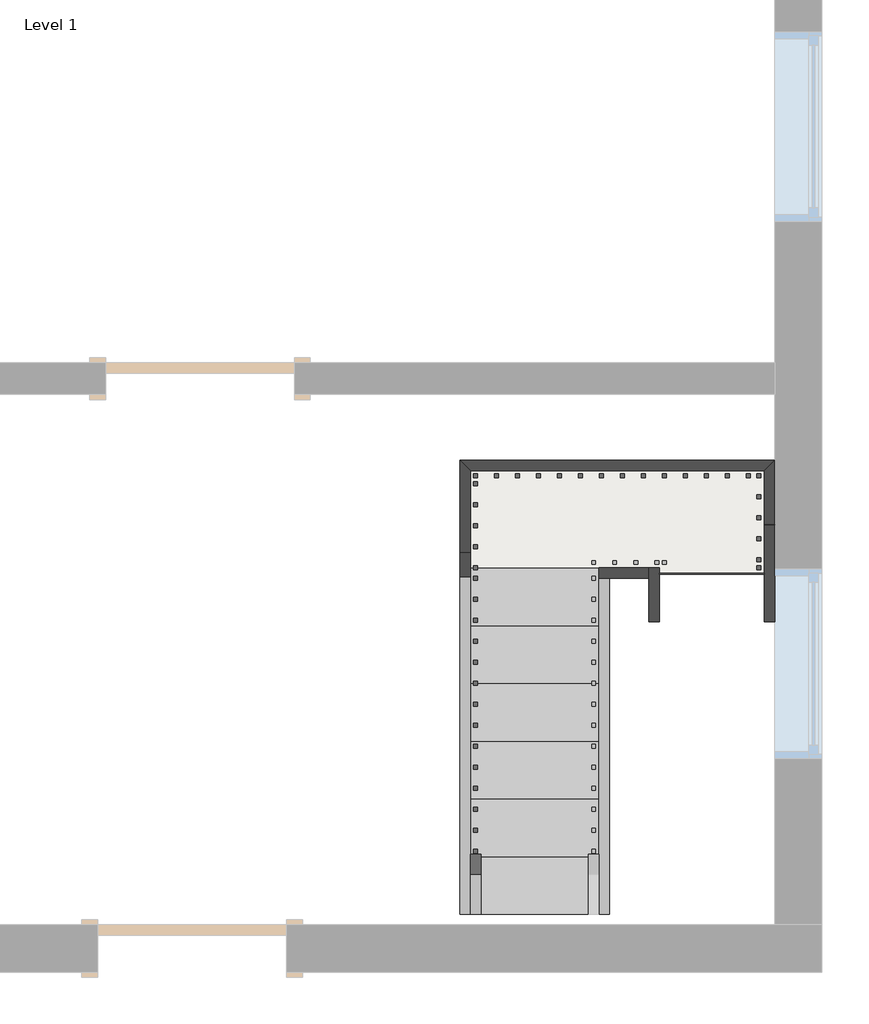
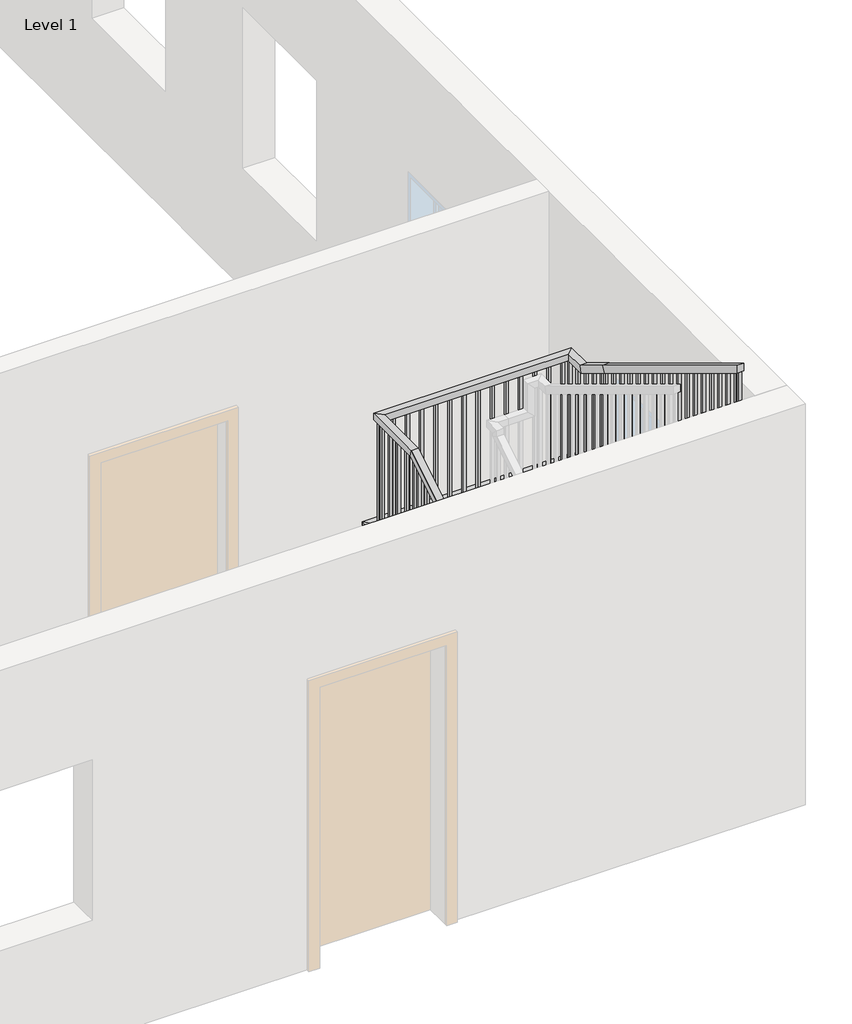
# One storey, part 2 of 2: 8 members, 2 stair flights, 1 railing, 1 slab.
"""IFC4 building model written with IfcOpenShell, lengths in millimetres."""

from ifc_helpers import new_model, si_unit, frame, origin, place, context, project, spatial, polyline, outline, extrude, faceted_brep, transform, mapped, element, save
from components import non_monolithic_landing_1ef36e8a, stair_flight_33de849b, stair_flight_7fe2dcbd

model = new_model("IFC4")

# Units and contexts
model_context = context("Model", 3, world=origin())
ifc_project = project(units=[si_unit("LENGTHUNIT", "METRE", prefix="MILLI")], contexts=[model_context])

# Site, building, storey
site = spatial("IfcSite", under=ifc_project)
building = spatial("IfcBuilding", under=site)
storey = spatial("IfcBuildingStorey", under=building, Name="Level 1", Elevation=0.0)

# Members
placement = place(None, origin())
element("IfcMember", 1, ObjectType="Stringer - 2\" Width", at=placement, inside=storey, context=model_context, shape_type="SweptSolid", body=[
    extrude(outline(polyline([(-4479.3424149, 0.0), (-4479.3424149, 212.114512), (-2747.8013597, 1261.5333333), (-2662.6469032, 956.7333333), (-4241.2569032, 0.0), (-4479.3424149, 0.0)])), frame((-1585.4629117, 0.0, 0.0), z_axis=(1.0, 0.0, 0.0), x_axis=(0.0, 1.0, 0.0)), (0.0, 0.0, 1.0), 50.8),
])
element("IfcMember", 2, ObjectType="Stringer - 2\" Width", at=placement, inside=storey, context=model_context, shape_type="SweptSolid", body=[
    extrude(outline(polyline([(-4479.3424149, 0.0), (-4479.3424149, 212.114512), (-2853.7424149, 1197.3266332), (-2853.7424149, 840.9178717), (-4241.2569032, 0.0), (-4479.3424149, 0.0)])), frame((-912.3629117, 0.0, 0.0), z_axis=(1.0, 0.0, 0.0), x_axis=(0.0, 1.0, 0.0)), (0.0, 0.0, 1.0), 50.8),
])
element("IfcMember", 3, ObjectType="Stringer - 2\" Width", at=placement, inside=storey, context=model_context, shape_type="SweptSolid", body=[
    extrude(outline(polyline([(-2578.6834702, 1261.5333333), (-2663.8379267, 956.7333333), (-4479.3424149, 2057.0390838), (-4479.3424149, 2413.4478453), (-2578.6834702, 1261.5333333)])), frame((-112.2629117, 0.0, 0.0), z_axis=(1.0, 0.0, 0.0), x_axis=(0.0, 1.0, 0.0)), (0.0, 0.0, 1.0), 50.8),
])
element("IfcMember", 4, ObjectType="Stringer - 2\" Width", at=placement, inside=storey, context=model_context, shape_type="SweptSolid", body=[
    extrude(outline(polyline([(-2802.9424149, 1397.4478453), (-2802.9424149, 1041.0390838), (-4479.3424149, 2057.0390838), (-4479.3424149, 2413.4478453), (-2802.9424149, 1397.4478453)])), frame((-671.0629117, 0.0, 0.0), z_axis=(1.0, 0.0, 0.0), x_axis=(0.0, 1.0, 0.0)), (0.0, 0.0, 1.0), 50.8),
])
element("IfcMember", 5, ObjectType="Stringer - 2\" Width", at=placement, inside=storey, context=model_context, shape_type="Brep", body=[
    faceted_brep([(-112.2629117, -2578.6834702, 1261.5333333), (-61.4629117, -2578.6834702, 1261.5333333), (-61.4629117, -2282.2424149, 1261.5333333), (-112.2629117, -2333.0424149, 1261.5333333), (-112.2629117, -2663.8379267, 956.7333333), (-112.2629117, -2333.0424149, 956.7333333), (-61.4629117, -2663.8379267, 956.7333333), (-61.4629117, -2282.2424149, 956.7333333)], [[[0, 1, 2, 3]], [[4, 0, 3, 5]], [[6, 4, 5, 7]], [[1, 6, 7, 2]], [[1, 0, 4, 6]], [[2, 7, 5, 3]]]),
])
element("IfcMember", 6, ObjectType="Stringer - 2\" Width", at=placement, inside=storey, context=model_context, shape_type="SweptSolid", body=[
    extrude(outline(polyline([(-61.4629117, -2282.2424149), (-112.2629117, -2333.0424149), (-1534.6629117, -2333.0424149), (-1585.4629117, -2282.2424149), (-61.4629117, -2282.2424149)])), frame((0.0, 0.0, 956.7333333), z_axis=(0.0, 0.0, 1.0), x_axis=(1.0, 0.0, 0.0)), (0.0, 0.0, 1.0), 304.8),
])
element("IfcMember", 7, ObjectType="Stringer - 2\" Width", at=placement, inside=storey, context=model_context, shape_type="Brep", body=[
    faceted_brep([(-1534.6629117, -2333.0424149, 1261.5333333), (-1585.4629117, -2282.2424149, 1261.5333333), (-1585.4629117, -2747.8013597, 1261.5333333), (-1534.6629117, -2747.8013597, 1261.5333333), (-1534.6629117, -2333.0424149, 956.7333333), (-1534.6629117, -2662.6469032, 956.7333333), (-1585.4629117, -2282.2424149, 956.7333333), (-1585.4629117, -2662.6469032, 956.7333333)], [[[0, 1, 2, 3]], [[4, 0, 3, 5]], [[6, 4, 5, 7]], [[1, 6, 7, 2]], [[1, 0, 4, 6]], [[2, 7, 5, 3]]]),
])
element("IfcMember", 8, ObjectType="Stringer - 2\" Width", at=placement, inside=storey, context=model_context, shape_type="SweptSolid", body=[
    extrude(outline(polyline([(-912.3629117, -2853.7424149), (-912.3629117, -2802.9424149), (-671.0629117, -2802.9424149), (-671.0629117, -2853.7424149), (-912.3629117, -2853.7424149)])), frame((0.0, 0.0, 956.7333333), z_axis=(0.0, 0.0, 1.0), x_axis=(1.0, 0.0, 0.0)), (0.0, 0.0, 1.0), 304.8),
])

# Railing
element("IfcRailing", 9, ObjectType="Handrail - Rectangular", at=placement, inside=storey, context=model_context, shape_type="SolidModel", body=[
    faceted_brep([(-1534.6629117, -4479.3424149, 1083.7333333), (-1534.6629117, -4479.3424149, 1024.3318731), (-1483.8629117, -4479.3424149, 1024.3318731), (-1483.8629117, -4479.3424149, 1083.7333333), (-1534.6629117, -2802.9424149, 2099.7333333), (-1534.6629117, -2788.7500055, 2048.9333333), (-1483.8629117, -2788.7500055, 2048.9333333), (-1483.8629117, -2802.9424149, 2099.7333333), (-1534.6629117, -2333.0424149, 2099.7333333), (-1534.6629117, -2333.0424149, 2048.9333333), (-1483.8629117, -2383.8424149, 2048.9333333), (-1483.8629117, -2383.8424149, 2099.7333333), (-112.2629117, -2333.0424149, 2099.7333333), (-112.2629117, -2333.0424149, 2048.9333333), (-163.0629117, -2383.8424149, 2048.9333333), (-163.0629117, -2383.8424149, 2099.7333333), (-112.2629117, -2523.5424149, 2099.7333333), (-112.2629117, -2537.7348244, 2048.9333333), (-163.0629117, -2537.7348244, 2048.9333333), (-163.0629117, -2523.5424149, 2099.7333333), (-112.2629117, -2802.9424149, 2269.0666667), (-112.2629117, -2829.2721421, 2225.6226168), (-163.0629117, -2829.2721421, 2225.6226168), (-163.0629117, -2802.9424149, 2269.0666667), (-112.2629117, -4479.3424149, 3285.0666667), (-163.0629117, -4479.3424149, 3285.0666667), (-163.0629117, -4479.3424149, 3225.6652064), (-112.2629117, -4479.3424149, 3225.6652064)], [[[0, 1, 2, 3]], [[1, 0, 4, 5]], [[2, 1, 5, 6]], [[3, 2, 6, 7]], [[0, 3, 7, 4]], [[5, 4, 8, 9]], [[6, 5, 9, 10]], [[7, 6, 10, 11]], [[4, 7, 11, 8]], [[9, 8, 12, 13]], [[10, 9, 13, 14]], [[11, 10, 14, 15]], [[8, 11, 15, 12]], [[13, 12, 16, 17]], [[14, 13, 17, 18]], [[15, 14, 18, 19]], [[12, 15, 19, 16]], [[17, 16, 20, 21]], [[18, 17, 21, 22]], [[19, 18, 22, 23]], [[16, 19, 23, 20]], [[24, 25, 26, 27]], [[21, 20, 24, 27]], [[22, 21, 27, 26]], [[23, 22, 26, 25]], [[20, 23, 25, 24]]]),
    extrude(outline(polyline([(-4419.0174149, 3189.1046004), (-4419.0174149, 2201.3333333), (-4438.0674149, 2201.3333333), (-4438.0674149, 3200.6500549), (-4419.0174149, 3189.1046004)])), frame((-147.1879117, 0.0, 0.0), z_axis=(1.0, 0.0, 0.0), x_axis=(0.0, 1.0, 0.0)), (0.0, 0.0, 1.0), 19.05),
    extrude(outline(polyline([(-4317.4174149, 3127.5288428), (-4317.4174149, 2201.3333333), (-4336.4674149, 2201.3333333), (-4336.4674149, 3139.0742973), (-4317.4174149, 3127.5288428)])), frame((-147.1879117, 0.0, 0.0), z_axis=(1.0, 0.0, 0.0), x_axis=(0.0, 1.0, 0.0)), (0.0, 0.0, 1.0), 19.05),
    extrude(outline(polyline([(-4215.8174149, 3065.9530852), (-4215.8174149, 2201.3333333), (-4234.8674149, 2201.3333333), (-4234.8674149, 3077.4985397), (-4215.8174149, 3065.9530852)])), frame((-147.1879117, 0.0, 0.0), z_axis=(1.0, 0.0, 0.0), x_axis=(0.0, 1.0, 0.0)), (0.0, 0.0, 1.0), 19.05),
    extrude(outline(polyline([(-4114.2174149, 3004.3773276), (-4114.2174149, 2032.0), (-4133.2674149, 2032.0), (-4133.2674149, 3015.9227822), (-4114.2174149, 3004.3773276)])), frame((-147.1879117, 0.0, 0.0), z_axis=(1.0, 0.0, 0.0), x_axis=(0.0, 1.0, 0.0)), (0.0, 0.0, 1.0), 19.05),
    extrude(outline(polyline([(-4012.6174149, 2942.80157), (-4012.6174149, 2032.0), (-4031.6674149, 2032.0), (-4031.6674149, 2954.3470246), (-4012.6174149, 2942.80157)])), frame((-147.1879117, 0.0, 0.0), z_axis=(1.0, 0.0, 0.0), x_axis=(0.0, 1.0, 0.0)), (0.0, 0.0, 1.0), 19.05),
    extrude(outline(polyline([(-3911.0174149, 2881.2258125), (-3911.0174149, 2032.0), (-3930.0674149, 2032.0), (-3930.0674149, 2892.771267), (-3911.0174149, 2881.2258125)])), frame((-147.1879117, 0.0, 0.0), z_axis=(1.0, 0.0, 0.0), x_axis=(0.0, 1.0, 0.0)), (0.0, 0.0, 1.0), 19.05),
    extrude(outline(polyline([(-3809.4174149, 2819.6500549), (-3809.4174149, 1862.6666667), (-3828.4674149, 1862.6666667), (-3828.4674149, 2831.1955094), (-3809.4174149, 2819.6500549)])), frame((-147.1879117, 0.0, 0.0), z_axis=(1.0, 0.0, 0.0), x_axis=(0.0, 1.0, 0.0)), (0.0, 0.0, 1.0), 19.05),
    extrude(outline(polyline([(-3707.8174149, 2758.0742973), (-3707.8174149, 1862.6666667), (-3726.8674149, 1862.6666667), (-3726.8674149, 2769.6197519), (-3707.8174149, 2758.0742973)])), frame((-147.1879117, 0.0, 0.0), z_axis=(1.0, 0.0, 0.0), x_axis=(0.0, 1.0, 0.0)), (0.0, 0.0, 1.0), 19.05),
    extrude(outline(polyline([(-3606.2174149, 2696.4985397), (-3606.2174149, 1693.3333333), (-3625.2674149, 1693.3333333), (-3625.2674149, 2708.0439943), (-3606.2174149, 2696.4985397)])), frame((-147.1879117, 0.0, 0.0), z_axis=(1.0, 0.0, 0.0), x_axis=(0.0, 1.0, 0.0)), (0.0, 0.0, 1.0), 19.05),
    extrude(outline(polyline([(-3504.6174149, 2634.9227822), (-3504.6174149, 1693.3333333), (-3523.6674149, 1693.3333333), (-3523.6674149, 2646.4682367), (-3504.6174149, 2634.9227822)])), frame((-147.1879117, 0.0, 0.0), z_axis=(1.0, 0.0, 0.0), x_axis=(0.0, 1.0, 0.0)), (0.0, 0.0, 1.0), 19.05),
    extrude(outline(polyline([(-3403.0174149, 2573.3470246), (-3403.0174149, 1693.3333333), (-3422.0674149, 1693.3333333), (-3422.0674149, 2584.8924791), (-3403.0174149, 2573.3470246)])), frame((-147.1879117, 0.0, 0.0), z_axis=(1.0, 0.0, 0.0), x_axis=(0.0, 1.0, 0.0)), (0.0, 0.0, 1.0), 19.05),
    extrude(outline(polyline([(-3301.4174149, 2511.771267), (-3301.4174149, 1524.0), (-3320.4674149, 1524.0), (-3320.4674149, 2523.3167216), (-3301.4174149, 2511.771267)])), frame((-147.1879117, 0.0, 0.0), z_axis=(1.0, 0.0, 0.0), x_axis=(0.0, 1.0, 0.0)), (0.0, 0.0, 1.0), 19.05),
    extrude(outline(polyline([(-3199.8174149, 2450.1955094), (-3199.8174149, 1524.0), (-3218.8674149, 1524.0), (-3218.8674149, 2461.740964), (-3199.8174149, 2450.1955094)])), frame((-147.1879117, 0.0, 0.0), z_axis=(1.0, 0.0, 0.0), x_axis=(0.0, 1.0, 0.0)), (0.0, 0.0, 1.0), 19.05),
    extrude(outline(polyline([(-3098.2174149, 2388.6197519), (-3098.2174149, 1524.0), (-3117.2674149, 1524.0), (-3117.2674149, 2400.1652064), (-3098.2174149, 2388.6197519)])), frame((-147.1879117, 0.0, 0.0), z_axis=(1.0, 0.0, 0.0), x_axis=(0.0, 1.0, 0.0)), (0.0, 0.0, 1.0), 19.05),
    extrude(outline(polyline([(-2996.6174149, 2327.0439943), (-2996.6174149, 1354.6666667), (-3015.6674149, 1354.6666667), (-3015.6674149, 2338.5894488), (-2996.6174149, 2327.0439943)])), frame((-147.1879117, 0.0, 0.0), z_axis=(1.0, 0.0, 0.0), x_axis=(0.0, 1.0, 0.0)), (0.0, 0.0, 1.0), 19.05),
    extrude(outline(polyline([(-2895.0174149, 2265.4682367), (-2895.0174149, 1354.6666667), (-2914.0674149, 1354.6666667), (-2914.0674149, 2277.0136913), (-2895.0174149, 2265.4682367)])), frame((-147.1879117, 0.0, 0.0), z_axis=(1.0, 0.0, 0.0), x_axis=(0.0, 1.0, 0.0)), (0.0, 0.0, 1.0), 19.05),
    extrude(outline(polyline([(-2755.3174149, 2180.80157), (-2755.3174149, 1185.3333333), (-2774.3674149, 1185.3333333), (-2774.3674149, 2192.3470246), (-2755.3174149, 2180.80157)])), frame((-147.1879117, 0.0, 0.0), z_axis=(1.0, 0.0, 0.0), x_axis=(0.0, 1.0, 0.0)), (0.0, 0.0, 1.0), 19.05),
    extrude(outline(polyline([(-2653.7174149, 2119.2258125), (-2653.7174149, 1185.3333333), (-2672.7674149, 1185.3333333), (-2672.7674149, 2130.771267), (-2653.7174149, 2119.2258125)])), frame((-147.1879117, 0.0, 0.0), z_axis=(1.0, 0.0, 0.0), x_axis=(0.0, 1.0, 0.0)), (0.0, 0.0, 1.0), 19.05),
    extrude(outline(polyline([(-2552.1174149, 2057.6500549), (-2552.1174149, 1185.3333333), (-2571.1674149, 1185.3333333), (-2571.1674149, 2069.1955094), (-2552.1174149, 2057.6500549)])), frame((-147.1879117, 0.0, 0.0), z_axis=(1.0, 0.0, 0.0), x_axis=(0.0, 1.0, 0.0)), (0.0, 0.0, 1.0), 19.05),
    extrude(outline(polyline([(-128.1379117, -2450.5174149), (-128.1379117, -2469.5674149), (-147.1879117, -2469.5674149), (-147.1879117, -2450.5174149), (-128.1379117, -2450.5174149)])), frame((0.0, 0.0, 1185.3333333), z_axis=(0.0, 0.0, 1.0), x_axis=(1.0, 0.0, 0.0)), (0.0, 0.0, 1.0), 863.6),
    extrude(outline(polyline([(-197.9879117, -2348.9174149), (-178.9379117, -2348.9174149), (-178.9379117, -2367.9674149), (-197.9879117, -2367.9674149), (-197.9879117, -2348.9174149)])), frame((0.0, 0.0, 1185.3333333), z_axis=(0.0, 0.0, 1.0), x_axis=(1.0, 0.0, 0.0)), (0.0, 0.0, 1.0), 863.6),
    extrude(outline(polyline([(-299.5879117, -2348.9174149), (-280.5379117, -2348.9174149), (-280.5379117, -2367.9674149), (-299.5879117, -2367.9674149), (-299.5879117, -2348.9174149)])), frame((0.0, 0.0, 1185.3333333), z_axis=(0.0, 0.0, 1.0), x_axis=(1.0, 0.0, 0.0)), (0.0, 0.0, 1.0), 863.6),
    extrude(outline(polyline([(-401.1879117, -2348.9174149), (-382.1379117, -2348.9174149), (-382.1379117, -2367.9674149), (-401.1879117, -2367.9674149), (-401.1879117, -2348.9174149)])), frame((0.0, 0.0, 1185.3333333), z_axis=(0.0, 0.0, 1.0), x_axis=(1.0, 0.0, 0.0)), (0.0, 0.0, 1.0), 863.6),
    extrude(outline(polyline([(-502.7879117, -2348.9174149), (-483.7379117, -2348.9174149), (-483.7379117, -2367.9674149), (-502.7879117, -2367.9674149), (-502.7879117, -2348.9174149)])), frame((0.0, 0.0, 1185.3333333), z_axis=(0.0, 0.0, 1.0), x_axis=(1.0, 0.0, 0.0)), (0.0, 0.0, 1.0), 863.6),
    extrude(outline(polyline([(-604.3879117, -2348.9174149), (-585.3379117, -2348.9174149), (-585.3379117, -2367.9674149), (-604.3879117, -2367.9674149), (-604.3879117, -2348.9174149)])), frame((0.0, 0.0, 1185.3333333), z_axis=(0.0, 0.0, 1.0), x_axis=(1.0, 0.0, 0.0)), (0.0, 0.0, 1.0), 863.6),
    extrude(outline(polyline([(-705.9879117, -2348.9174149), (-686.9379117, -2348.9174149), (-686.9379117, -2367.9674149), (-705.9879117, -2367.9674149), (-705.9879117, -2348.9174149)])), frame((0.0, 0.0, 1185.3333333), z_axis=(0.0, 0.0, 1.0), x_axis=(1.0, 0.0, 0.0)), (0.0, 0.0, 1.0), 863.6),
    extrude(outline(polyline([(-807.5879117, -2348.9174149), (-788.5379117, -2348.9174149), (-788.5379117, -2367.9674149), (-807.5879117, -2367.9674149), (-807.5879117, -2348.9174149)])), frame((0.0, 0.0, 1185.3333333), z_axis=(0.0, 0.0, 1.0), x_axis=(1.0, 0.0, 0.0)), (0.0, 0.0, 1.0), 863.6),
    extrude(outline(polyline([(-909.1879117, -2348.9174149), (-890.1379117, -2348.9174149), (-890.1379117, -2367.9674149), (-909.1879117, -2367.9674149), (-909.1879117, -2348.9174149)])), frame((0.0, 0.0, 1185.3333333), z_axis=(0.0, 0.0, 1.0), x_axis=(1.0, 0.0, 0.0)), (0.0, 0.0, 1.0), 863.6),
    extrude(outline(polyline([(-1010.7879117, -2348.9174149), (-991.7379117, -2348.9174149), (-991.7379117, -2367.9674149), (-1010.7879117, -2367.9674149), (-1010.7879117, -2348.9174149)])), frame((0.0, 0.0, 1185.3333333), z_axis=(0.0, 0.0, 1.0), x_axis=(1.0, 0.0, 0.0)), (0.0, 0.0, 1.0), 863.6),
    extrude(outline(polyline([(-1112.3879117, -2348.9174149), (-1093.3379117, -2348.9174149), (-1093.3379117, -2367.9674149), (-1112.3879117, -2367.9674149), (-1112.3879117, -2348.9174149)])), frame((0.0, 0.0, 1185.3333333), z_axis=(0.0, 0.0, 1.0), x_axis=(1.0, 0.0, 0.0)), (0.0, 0.0, 1.0), 863.6),
    extrude(outline(polyline([(-1213.9879117, -2348.9174149), (-1194.9379117, -2348.9174149), (-1194.9379117, -2367.9674149), (-1213.9879117, -2367.9674149), (-1213.9879117, -2348.9174149)])), frame((0.0, 0.0, 1185.3333333), z_axis=(0.0, 0.0, 1.0), x_axis=(1.0, 0.0, 0.0)), (0.0, 0.0, 1.0), 863.6),
    extrude(outline(polyline([(-1315.5879117, -2348.9174149), (-1296.5379117, -2348.9174149), (-1296.5379117, -2367.9674149), (-1315.5879117, -2367.9674149), (-1315.5879117, -2348.9174149)])), frame((0.0, 0.0, 1185.3333333), z_axis=(0.0, 0.0, 1.0), x_axis=(1.0, 0.0, 0.0)), (0.0, 0.0, 1.0), 863.6),
    extrude(outline(polyline([(-1417.1879117, -2348.9174149), (-1398.1379117, -2348.9174149), (-1398.1379117, -2367.9674149), (-1417.1879117, -2367.9674149), (-1417.1879117, -2348.9174149)])), frame((0.0, 0.0, 1185.3333333), z_axis=(0.0, 0.0, 1.0), x_axis=(1.0, 0.0, 0.0)), (0.0, 0.0, 1.0), 863.6),
    extrude(outline(polyline([(-1518.7879117, -2406.0674149), (-1518.7879117, -2387.0174149), (-1499.7379117, -2387.0174149), (-1499.7379117, -2406.0674149), (-1518.7879117, -2406.0674149)])), frame((0.0, 0.0, 1185.3333333), z_axis=(0.0, 0.0, 1.0), x_axis=(1.0, 0.0, 0.0)), (0.0, 0.0, 1.0), 863.6),
    extrude(outline(polyline([(-1518.7879117, -2507.6674149), (-1518.7879117, -2488.6174149), (-1499.7379117, -2488.6174149), (-1499.7379117, -2507.6674149), (-1518.7879117, -2507.6674149)])), frame((0.0, 0.0, 1185.3333333), z_axis=(0.0, 0.0, 1.0), x_axis=(1.0, 0.0, 0.0)), (0.0, 0.0, 1.0), 863.6),
    extrude(outline(polyline([(-1518.7879117, -2609.2674149), (-1518.7879117, -2590.2174149), (-1499.7379117, -2590.2174149), (-1499.7379117, -2609.2674149), (-1518.7879117, -2609.2674149)])), frame((0.0, 0.0, 1185.3333333), z_axis=(0.0, 0.0, 1.0), x_axis=(1.0, 0.0, 0.0)), (0.0, 0.0, 1.0), 863.6),
    extrude(outline(polyline([(-1518.7879117, -2710.8674149), (-1518.7879117, -2691.8174149), (-1499.7379117, -2691.8174149), (-1499.7379117, -2710.8674149), (-1518.7879117, -2710.8674149)])), frame((0.0, 0.0, 1185.3333333), z_axis=(0.0, 0.0, 1.0), x_axis=(1.0, 0.0, 0.0)), (0.0, 0.0, 1.0), 863.6),
    extrude(outline(polyline([(-2844.2174149, 2015.3167216), (-2844.2174149, 1016.0), (-2863.2674149, 1016.0), (-2863.2674149, 2003.771267), (-2844.2174149, 2015.3167216)])), frame((-1518.7879117, 0.0, 0.0), z_axis=(1.0, 0.0, 0.0), x_axis=(0.0, 1.0, 0.0)), (0.0, 0.0, 1.0), 19.05),
    extrude(outline(polyline([(-2945.8174149, 1953.740964), (-2945.8174149, 1016.0), (-2964.8674149, 1016.0), (-2964.8674149, 1942.1955094), (-2945.8174149, 1953.740964)])), frame((-1518.7879117, 0.0, 0.0), z_axis=(1.0, 0.0, 0.0), x_axis=(0.0, 1.0, 0.0)), (0.0, 0.0, 1.0), 19.05),
    extrude(outline(polyline([(-3047.4174149, 1892.1652064), (-3047.4174149, 1016.0), (-3066.4674149, 1016.0), (-3066.4674149, 1880.6197519), (-3047.4174149, 1892.1652064)])), frame((-1518.7879117, 0.0, 0.0), z_axis=(1.0, 0.0, 0.0), x_axis=(0.0, 1.0, 0.0)), (0.0, 0.0, 1.0), 19.05),
    extrude(outline(polyline([(-3149.0174149, 1830.5894488), (-3149.0174149, 846.6666667), (-3168.0674149, 846.6666667), (-3168.0674149, 1819.0439943), (-3149.0174149, 1830.5894488)])), frame((-1518.7879117, 0.0, 0.0), z_axis=(1.0, 0.0, 0.0), x_axis=(0.0, 1.0, 0.0)), (0.0, 0.0, 1.0), 19.05),
    extrude(outline(polyline([(-3250.6174149, 1769.0136913), (-3250.6174149, 846.6666667), (-3269.6674149, 846.6666667), (-3269.6674149, 1757.4682367), (-3250.6174149, 1769.0136913)])), frame((-1518.7879117, 0.0, 0.0), z_axis=(1.0, 0.0, 0.0), x_axis=(0.0, 1.0, 0.0)), (0.0, 0.0, 1.0), 19.05),
    extrude(outline(polyline([(-3352.2174149, 1707.4379337), (-3352.2174149, 846.6666667), (-3371.2674149, 846.6666667), (-3371.2674149, 1695.8924791), (-3352.2174149, 1707.4379337)])), frame((-1518.7879117, 0.0, 0.0), z_axis=(1.0, 0.0, 0.0), x_axis=(0.0, 1.0, 0.0)), (0.0, 0.0, 1.0), 19.05),
    extrude(outline(polyline([(-3453.8174149, 1645.8621761), (-3453.8174149, 677.3333333), (-3472.8674149, 677.3333333), (-3472.8674149, 1634.3167216), (-3453.8174149, 1645.8621761)])), frame((-1518.7879117, 0.0, 0.0), z_axis=(1.0, 0.0, 0.0), x_axis=(0.0, 1.0, 0.0)), (0.0, 0.0, 1.0), 19.05),
    extrude(outline(polyline([(-3555.4174149, 1584.2864185), (-3555.4174149, 677.3333333), (-3574.4674149, 677.3333333), (-3574.4674149, 1572.740964), (-3555.4174149, 1584.2864185)])), frame((-1518.7879117, 0.0, 0.0), z_axis=(1.0, 0.0, 0.0), x_axis=(0.0, 1.0, 0.0)), (0.0, 0.0, 1.0), 19.05),
    extrude(outline(polyline([(-3657.0174149, 1522.710661), (-3657.0174149, 508.0), (-3676.0674149, 508.0), (-3676.0674149, 1511.1652064), (-3657.0174149, 1522.710661)])), frame((-1518.7879117, 0.0, 0.0), z_axis=(1.0, 0.0, 0.0), x_axis=(0.0, 1.0, 0.0)), (0.0, 0.0, 1.0), 19.05),
    extrude(outline(polyline([(-3758.6174149, 1461.1349034), (-3758.6174149, 508.0), (-3777.6674149, 508.0), (-3777.6674149, 1449.5894488), (-3758.6174149, 1461.1349034)])), frame((-1518.7879117, 0.0, 0.0), z_axis=(1.0, 0.0, 0.0), x_axis=(0.0, 1.0, 0.0)), (0.0, 0.0, 1.0), 19.05),
    extrude(outline(polyline([(-3860.2174149, 1399.5591458), (-3860.2174149, 508.0), (-3879.2674149, 508.0), (-3879.2674149, 1388.0136913), (-3860.2174149, 1399.5591458)])), frame((-1518.7879117, 0.0, 0.0), z_axis=(1.0, 0.0, 0.0), x_axis=(0.0, 1.0, 0.0)), (0.0, 0.0, 1.0), 19.05),
    extrude(outline(polyline([(-3961.8174149, 1337.9833882), (-3961.8174149, 338.6666667), (-3980.8674149, 338.6666667), (-3980.8674149, 1326.4379337), (-3961.8174149, 1337.9833882)])), frame((-1518.7879117, 0.0, 0.0), z_axis=(1.0, 0.0, 0.0), x_axis=(0.0, 1.0, 0.0)), (0.0, 0.0, 1.0), 19.05),
    extrude(outline(polyline([(-4063.4174149, 1276.4076307), (-4063.4174149, 338.6666667), (-4082.4674149, 338.6666667), (-4082.4674149, 1264.8621761), (-4063.4174149, 1276.4076307)])), frame((-1518.7879117, 0.0, 0.0), z_axis=(1.0, 0.0, 0.0), x_axis=(0.0, 1.0, 0.0)), (0.0, 0.0, 1.0), 19.05),
    extrude(outline(polyline([(-4165.0174149, 1214.8318731), (-4165.0174149, 338.6666667), (-4184.0674149, 338.6666667), (-4184.0674149, 1203.2864185), (-4165.0174149, 1214.8318731)])), frame((-1518.7879117, 0.0, 0.0), z_axis=(1.0, 0.0, 0.0), x_axis=(0.0, 1.0, 0.0)), (0.0, 0.0, 1.0), 19.05),
    extrude(outline(polyline([(-4266.6174149, 1153.2561155), (-4266.6174149, 169.3333333), (-4285.6674149, 169.3333333), (-4285.6674149, 1141.710661), (-4266.6174149, 1153.2561155)])), frame((-1518.7879117, 0.0, 0.0), z_axis=(1.0, 0.0, 0.0), x_axis=(0.0, 1.0, 0.0)), (0.0, 0.0, 1.0), 19.05),
    extrude(outline(polyline([(-4368.2174149, 1091.6803579), (-4368.2174149, 169.3333333), (-4387.2674149, 169.3333333), (-4387.2674149, 1080.1349034), (-4368.2174149, 1091.6803579)])), frame((-1518.7879117, 0.0, 0.0), z_axis=(1.0, 0.0, 0.0), x_axis=(0.0, 1.0, 0.0)), (0.0, 0.0, 1.0), 19.05),
    extrude(outline(polyline([(-2793.4174149, 2203.8924791), (-2793.4174149, 1185.3333333), (-2812.4674149, 1185.3333333), (-2812.4674149, 2215.4379337), (-2793.4174149, 2203.8924791)])), frame((-147.1879117, 0.0, 0.0), z_axis=(1.0, 0.0, 0.0), x_axis=(0.0, 1.0, 0.0)), (0.0, 0.0, 1.0), 19.05),
    extrude(outline(polyline([(-147.1879117, -2348.9174149), (-128.1379117, -2348.9174149), (-128.1379117, -2367.9674149), (-147.1879117, -2367.9674149), (-147.1879117, -2348.9174149)])), frame((0.0, 0.0, 1185.3333333), z_axis=(0.0, 0.0, 1.0), x_axis=(1.0, 0.0, 0.0)), (0.0, 0.0, 1.0), 863.6),
    extrude(outline(polyline([(-1518.7879117, -2367.9674149), (-1518.7879117, -2348.9174149), (-1499.7379117, -2348.9174149), (-1499.7379117, -2367.9674149), (-1518.7879117, -2367.9674149)])), frame((0.0, 0.0, 1185.3333333), z_axis=(0.0, 0.0, 1.0), x_axis=(1.0, 0.0, 0.0)), (0.0, 0.0, 1.0), 863.6),
    extrude(outline(polyline([(-2793.4174149, 2046.1046004), (-2793.4174149, 1185.3333333), (-2812.4674149, 1185.3333333), (-2812.4674149, 2034.5591458), (-2793.4174149, 2046.1046004)])), frame((-1518.7879117, 0.0, 0.0), z_axis=(1.0, 0.0, 0.0), x_axis=(0.0, 1.0, 0.0)), (0.0, 0.0, 1.0), 19.05),
    extrude(outline(polyline([(-4460.2924149, 3214.1197519), (-4460.2924149, 2201.3333333), (-4479.3424149, 2201.3333333), (-4479.3424149, 3225.6652064), (-4460.2924149, 3214.1197519)])), frame((-147.1879117, 0.0, 0.0), z_axis=(1.0, 0.0, 0.0), x_axis=(0.0, 1.0, 0.0)), (0.0, 0.0, 1.0), 19.05),
    extrude(outline(polyline([(-4460.2924149, 1035.8773276), (-4460.2924149, 169.3333333), (-4479.3424149, 169.3333333), (-4479.3424149, 1024.3318731), (-4460.2924149, 1035.8773276)])), frame((-1518.7879117, 0.0, 0.0), z_axis=(1.0, 0.0, 0.0), x_axis=(0.0, 1.0, 0.0)), (0.0, 0.0, 1.0), 19.05),
])

# Slab
non_monolithic_landing_shape = non_monolithic_landing_1ef36e8a(model_context)
element("IfcSlab", 10, ObjectType="Non-Monolithic Landing", at=placement, inside=storey, context=model_context, shape_type="MappedRepresentation", body=[
    mapped(non_monolithic_landing_shape, transform((0.0, 0.0, 0.0), x_axis=(1.0, 0.0, 0.0), y_axis=(0.0, 1.0, 0.0), z_axis=(0.0, 0.0, 1.0))),
])

# Stair flights
stair_flight_shape = stair_flight_33de849b(model_context)
element("IfcStairFlight", 11, ObjectType="2\" Tread 1\" Nosing 1/4\" Riser", at=placement, inside=storey, context=model_context, shape_type="MappedRepresentation", body=[
    mapped(stair_flight_shape, transform((0.0, 0.0, 0.0), x_axis=(1.0, 0.0, 0.0), y_axis=(0.0, 1.0, 0.0), z_axis=(0.0, 0.0, 1.0))),
])
stair_flight_2_shape = stair_flight_7fe2dcbd(model_context)
element("IfcStairFlight", 12, ObjectType="2\" Tread 1\" Nosing 1/4\" Riser", at=placement, inside=storey, context=model_context, shape_type="MappedRepresentation", body=[
    mapped(stair_flight_2_shape, transform((0.0, 0.0, 0.0), x_axis=(1.0, 0.0, 0.0), y_axis=(0.0, 1.0, 0.0), z_axis=(0.0, 0.0, 1.0))),
])

save(model, "model.ifc")

# Revit data of these elements
# Type "Handrail - Rectangular"
#   Assembly Code = "C2010400"
#   built-in parameter 1008612 = 0.0416667 (stored number, unit not read)
#   built-in parameter 1008611 = 0.0416667 (stored number, unit not read)
#   built-in parameter 1008609 = 0.333333 (stored number, unit not read)
#   built-in parameter 1008604 = 0.166667 (stored number, unit not read)
#   built-in parameter 1008603 = 0.166667 (stored number, unit not read)
#   Railing Height = 3' - 0"
#   built-in parameter 1008630 = 2
#   built-in parameter 1008610 = 2
#   built-in parameter 1008618 = Baluster - Square : 3/4"
# Elements 1, 2, 3, 4, 5, 6, 7, 8 (IfcMember, "Stringer - 2\" Width")
#   Phase Created = New Construction
# Element 9 (IfcRailing, "Handrail - Rectangular")
#   Phase Created = New Construction
# Element 10 (IfcSlab, "Non-Monolithic Landing")
#   Phase Created = New Construction
# Elements 11, 12 (IfcStairFlight, "2\" Tread 1\" Nosing 1/4\" Riser")
#   Phase Created = New Construction
